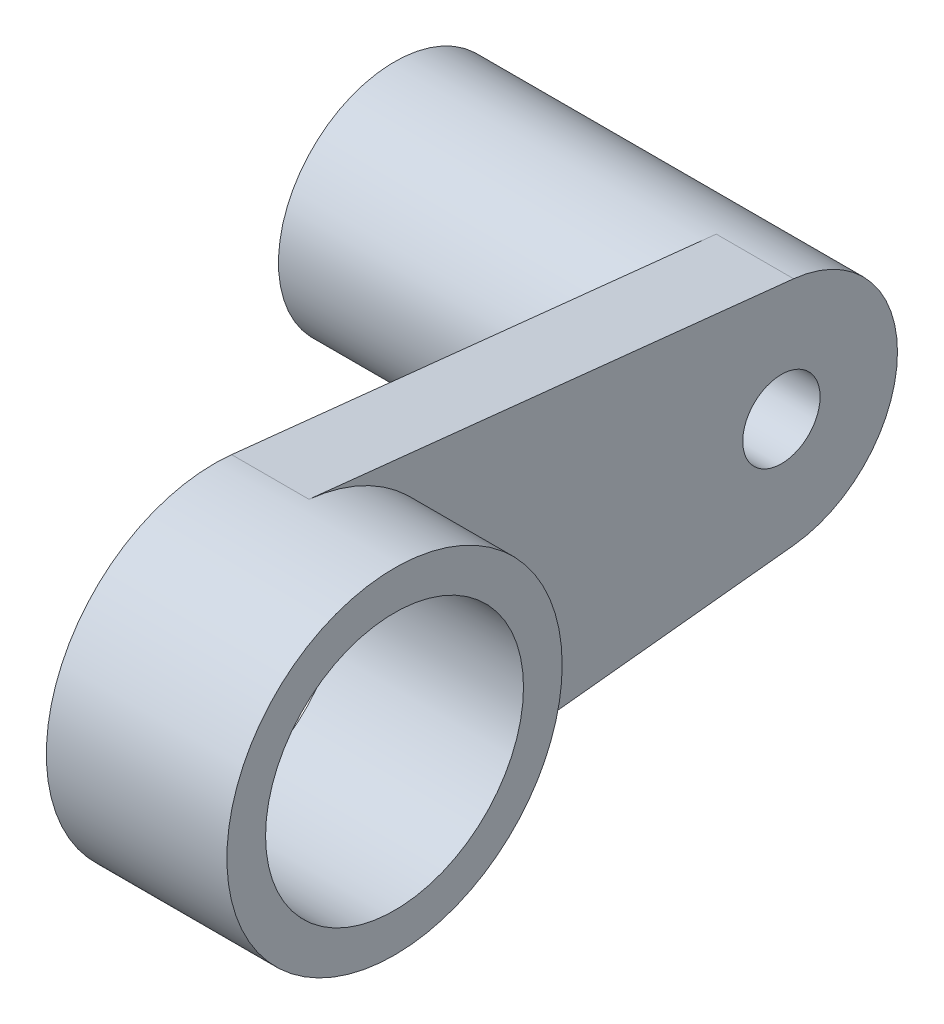
ISO-10303-21;
HEADER;
FILE_DESCRIPTION(('STEP AP214'),'2;1');
FILE_NAME('part.step','',(''),(''),'','','');
FILE_SCHEMA(('AUTOMOTIVE_DESIGN { 1 0 10303 214 1 1 1 1 }'));
ENDSEC;
DATA;
#1=APPLICATION_CONTEXT('core data for automotive mechanical design processes');
#2=APPLICATION_PROTOCOL_DEFINITION('international standard','automotive_design',2000,#1);
#3=PRODUCT_CONTEXT('',#1,'mechanical');
#4=PRODUCT('Part','Part','',(#3));
#5=PRODUCT_RELATED_PRODUCT_CATEGORY('part','',(#4));
#6=PRODUCT_DEFINITION_FORMATION('','',#4);
#7=PRODUCT_DEFINITION_CONTEXT('part definition',#1,'design');
#8=PRODUCT_DEFINITION('design','',#6,#7);
#9=PRODUCT_DEFINITION_SHAPE('','',#8);
#10=(LENGTH_UNIT() NAMED_UNIT(*) SI_UNIT(.MILLI.,.METRE.));
#11=(NAMED_UNIT(*) PLANE_ANGLE_UNIT() SI_UNIT($,.RADIAN.));
#12=(NAMED_UNIT(*) SI_UNIT($,.STERADIAN.) SOLID_ANGLE_UNIT());
#13=UNCERTAINTY_MEASURE_WITH_UNIT(LENGTH_MEASURE(1.E-05),#10,'distance_accuracy_value','');
#14=(GEOMETRIC_REPRESENTATION_CONTEXT(3) GLOBAL_UNCERTAINTY_ASSIGNED_CONTEXT((#13)) GLOBAL_UNIT_ASSIGNED_CONTEXT((#10,
#11,#12)) REPRESENTATION_CONTEXT('',''));
#15=CARTESIAN_POINT('',(0.,0.,0.));
#16=DIRECTION('',(0.,0.,1.));
#17=DIRECTION('',(1.,0.,0.));
#18=AXIS2_PLACEMENT_3D('',#15,#16,#17);
#19=CARTESIAN_POINT('',(14.,0.,0.));
#20=DIRECTION('',(-1.,0.,0.));
#21=DIRECTION('',(0.,0.,1.));
#22=AXIS2_PLACEMENT_3D('',#19,#20,#21);
#23=CYLINDRICAL_SURFACE('',#22,13.);
#24=CARTESIAN_POINT('',(14.,0.,0.));
#25=DIRECTION('',(1.,0.,0.));
#26=DIRECTION('',(0.,0.,-1.));
#27=AXIS2_PLACEMENT_3D('',#24,#25,#26);
#28=CIRCLE('',#27,13.);
#29=CARTESIAN_POINT('',(14.,0.,-13.));
#30=VERTEX_POINT('',#29);
#31=EDGE_CURVE('E11',#30,#30,#28,.T.);
#32=ORIENTED_EDGE('',*,*,#31,.F.);
#33=EDGE_LOOP('',(#32));
#34=FACE_BOUND('',#33,.T.);
#35=DIRECTION('',(-1.,0.,0.));
#36=VECTOR('',#35,1.);
#37=CARTESIAN_POINT('',(6.,-12.9277772189466,-1.36842105263158));
#38=LINE('',#37,#36);
#39=CARTESIAN_POINT('',(6.,-12.9277772189466,-1.36842105263158));
#40=VERTEX_POINT('',#39);
#41=CARTESIAN_POINT('',(0.,-12.9277772189466,-1.36842105263158));
#42=VERTEX_POINT('',#41);
#43=EDGE_CURVE('E63',#40,#42,#38,.T.);
#44=ORIENTED_EDGE('',*,*,#43,.F.);
#45=CARTESIAN_POINT('',(6.,0.,0.));
#46=DIRECTION('',(1.,0.,0.));
#47=DIRECTION('',(0.,0.,-1.));
#48=AXIS2_PLACEMENT_3D('',#45,#46,#47);
#49=CIRCLE('',#48,13.);
#50=CARTESIAN_POINT('',(6.,12.9277772189466,-1.36842105263158));
#51=VERTEX_POINT('',#50);
#52=EDGE_CURVE('E59',#40,#51,#49,.T.);
#53=ORIENTED_EDGE('',*,*,#52,.T.);
#54=DIRECTION('',(-1.,0.,0.));
#55=VECTOR('',#54,1.);
#56=CARTESIAN_POINT('',(6.,12.9277772189466,-1.36842105263158));
#57=LINE('',#56,#55);
#58=CARTESIAN_POINT('',(0.,12.9277772189466,-1.36842105263158));
#59=VERTEX_POINT('',#58);
#60=EDGE_CURVE('E111',#51,#59,#57,.T.);
#61=ORIENTED_EDGE('',*,*,#60,.T.);
#62=CARTESIAN_POINT('',(0.,0.,0.));
#63=DIRECTION('',(1.,0.,0.));
#64=DIRECTION('',(0.,0.,-1.));
#65=AXIS2_PLACEMENT_3D('',#62,#63,#64);
#66=CIRCLE('',#65,13.);
#67=EDGE_CURVE('E116',#59,#42,#66,.T.);
#68=ORIENTED_EDGE('',*,*,#67,.T.);
#69=EDGE_LOOP('',(#44,#53,#61,#68));
#70=FACE_BOUND('',#69,.T.);
#71=ADVANCED_FACE('F41',(#34,#70),#23,.T.);
#72=CARTESIAN_POINT('',(14.,0.,0.));
#73=DIRECTION('',(-1.,0.,0.));
#74=DIRECTION('',(0.,0.,1.));
#75=AXIS2_PLACEMENT_3D('',#72,#73,#74);
#76=CYLINDRICAL_SURFACE('',#75,10.);
#77=CARTESIAN_POINT('',(14.,0.,0.));
#78=DIRECTION('',(1.,0.,0.));
#79=DIRECTION('',(0.,0.,-1.));
#80=AXIS2_PLACEMENT_3D('',#77,#78,#79);
#81=CIRCLE('',#80,10.);
#82=CARTESIAN_POINT('',(14.,0.,-10.));
#83=VERTEX_POINT('',#82);
#84=EDGE_CURVE('E49',#83,#83,#81,.T.);
#85=ORIENTED_EDGE('',*,*,#84,.T.);
#86=EDGE_LOOP('',(#85));
#87=FACE_BOUND('',#86,.T.);
#88=CARTESIAN_POINT('',(0.,0.,0.));
#89=DIRECTION('',(1.,0.,0.));
#90=DIRECTION('',(0.,0.,-1.));
#91=AXIS2_PLACEMENT_3D('',#88,#89,#90);
#92=CIRCLE('',#91,10.);
#93=CARTESIAN_POINT('',(0.,0.,-10.));
#94=VERTEX_POINT('',#93);
#95=EDGE_CURVE('E118',#94,#94,#92,.T.);
#96=ORIENTED_EDGE('',*,*,#95,.F.);
#97=EDGE_LOOP('',(#96));
#98=FACE_BOUND('',#97,.T.);
#99=ADVANCED_FACE('F43',(#87,#98),#76,.F.);
#100=CARTESIAN_POINT('',(14.,0.,0.));
#101=DIRECTION('',(1.,0.,0.));
#102=DIRECTION('',(0.,0.,-1.));
#103=AXIS2_PLACEMENT_3D('',#100,#101,#102);
#104=PLANE('',#103);
#105=ORIENTED_EDGE('',*,*,#84,.F.);
#106=EDGE_LOOP('',(#105));
#107=FACE_BOUND('',#106,.T.);
#108=ORIENTED_EDGE('',*,*,#31,.T.);
#109=EDGE_LOOP('',(#108));
#110=FACE_BOUND('',#109,.T.);
#111=ADVANCED_FACE('F160',(#107,#110),#104,.T.);
#112=CARTESIAN_POINT('',(0.,0.,0.));
#113=DIRECTION('',(1.,0.,0.));
#114=DIRECTION('',(0.,0.,-1.));
#115=AXIS2_PLACEMENT_3D('',#112,#113,#114);
#116=PLANE('',#115);
#117=ORIENTED_EDGE('',*,*,#95,.T.);
#118=EDGE_LOOP('',(#117));
#119=FACE_BOUND('',#118,.T.);
#120=DIRECTION('',(0.,-0.105263157894737,-0.994444401457431));
#121=VECTOR('',#120,1.);
#122=CARTESIAN_POINT('',(0.,12.9277772189466,-1.36842105263158));
#123=LINE('',#122,#121);
#124=CARTESIAN_POINT('',(0.,8.94999961311688,-38.9473684210526));
#125=VERTEX_POINT('',#124);
#126=EDGE_CURVE('E90',#59,#125,#123,.T.);
#127=ORIENTED_EDGE('',*,*,#126,.T.);
#128=CARTESIAN_POINT('',(0.,0.,-38.));
#129=DIRECTION('',(1.,0.,0.));
#130=DIRECTION('',(0.,0.,-1.));
#131=AXIS2_PLACEMENT_3D('',#128,#129,#130);
#132=CIRCLE('',#131,9.);
#133=CARTESIAN_POINT('',(0.,-8.94999961311688,-38.9473684210526));
#134=VERTEX_POINT('',#133);
#135=EDGE_CURVE('E82',#125,#134,#132,.T.);
#136=ORIENTED_EDGE('',*,*,#135,.T.);
#137=DIRECTION('',(0.,-0.105263157894737,0.994444401457431));
#138=VECTOR('',#137,1.);
#139=CARTESIAN_POINT('',(0.,-12.9277772189466,-1.36842105263158));
#140=LINE('',#139,#138);
#141=EDGE_CURVE('E87',#134,#42,#140,.T.);
#142=ORIENTED_EDGE('',*,*,#141,.T.);
#143=ORIENTED_EDGE('',*,*,#67,.F.);
#144=EDGE_LOOP('',(#127,#136,#142,#143));
#145=FACE_BOUND('',#144,.T.);
#146=ADVANCED_FACE('F81',(#119,#145),#116,.F.);
#147=CARTESIAN_POINT('',(6.,-12.9277772189466,-1.36842105263158));
#148=DIRECTION('',(0.,-0.994444401457431,-0.105263157894737));
#149=DIRECTION('',(0.,0.105263157894737,-0.994444401457431));
#150=AXIS2_PLACEMENT_3D('',#147,#148,#149);
#151=PLANE('',#150);
#152=ORIENTED_EDGE('',*,*,#141,.F.);
#153=DIRECTION('',(-1.,0.,0.));
#154=VECTOR('',#153,1.);
#155=CARTESIAN_POINT('',(6.,-8.94999961311688,-38.9473684210526));
#156=LINE('',#155,#154);
#157=CARTESIAN_POINT('',(6.,-8.94999961311688,-38.9473684210526));
#158=VERTEX_POINT('',#157);
#159=EDGE_CURVE('E96',#158,#134,#156,.T.);
#160=ORIENTED_EDGE('',*,*,#159,.F.);
#161=DIRECTION('',(0.,-0.105263157894737,0.994444401457431));
#162=VECTOR('',#161,1.);
#163=CARTESIAN_POINT('',(6.,-12.9277772189466,-1.36842105263158));
#164=LINE('',#163,#162);
#165=EDGE_CURVE('E126',#158,#40,#164,.T.);
#166=ORIENTED_EDGE('',*,*,#165,.T.);
#167=ORIENTED_EDGE('',*,*,#43,.T.);
#168=EDGE_LOOP('',(#152,#160,#166,#167));
#169=FACE_BOUND('',#168,.T.);
#170=ADVANCED_FACE('F104',(#169),#151,.T.);
#171=CARTESIAN_POINT('',(6.,0.,-38.));
#172=DIRECTION('',(-1.,0.,0.));
#173=DIRECTION('',(0.,0.,1.));
#174=AXIS2_PLACEMENT_3D('',#171,#172,#173);
#175=CYLINDRICAL_SURFACE('',#174,9.);
#176=ORIENTED_EDGE('',*,*,#159,.T.);
#177=ORIENTED_EDGE('',*,*,#135,.F.);
#178=DIRECTION('',(-1.,0.,0.));
#179=VECTOR('',#178,1.);
#180=CARTESIAN_POINT('',(6.,8.94999961311688,-38.9473684210526));
#181=LINE('',#180,#179);
#182=CARTESIAN_POINT('',(6.,8.94999961311688,-38.9473684210526));
#183=VERTEX_POINT('',#182);
#184=EDGE_CURVE('E103',#183,#125,#181,.T.);
#185=ORIENTED_EDGE('',*,*,#184,.F.);
#186=CARTESIAN_POINT('',(6.,0.,-38.));
#187=DIRECTION('',(1.,0.,0.));
#188=DIRECTION('',(0.,0.,-1.));
#189=AXIS2_PLACEMENT_3D('',#186,#187,#188);
#190=CIRCLE('',#189,9.);
#191=EDGE_CURVE('E97',#158,#183,#190,.T.);
#192=ORIENTED_EDGE('',*,*,#191,.F.);
#193=EDGE_LOOP('',(#176,#177,#185,#192));
#194=FACE_BOUND('',#193,.T.);
#195=CARTESIAN_POINT('',(-24.,0.,-38.));
#196=DIRECTION('',(1.,0.,0.));
#197=DIRECTION('',(0.,0.,-1.));
#198=AXIS2_PLACEMENT_3D('',#195,#196,#197);
#199=CIRCLE('',#198,9.);
#200=CARTESIAN_POINT('',(-24.,0.,-47.));
#201=VERTEX_POINT('',#200);
#202=EDGE_CURVE('E91',#201,#201,#199,.T.);
#203=ORIENTED_EDGE('',*,*,#202,.T.);
#204=EDGE_LOOP('',(#203));
#205=FACE_BOUND('',#204,.T.);
#206=ADVANCED_FACE('F100',(#194,#205),#175,.T.);
#207=CARTESIAN_POINT('',(6.,12.9277772189466,-1.36842105263158));
#208=DIRECTION('',(0.,0.994444401457431,-0.105263157894737));
#209=DIRECTION('',(0.,0.105263157894737,0.994444401457431));
#210=AXIS2_PLACEMENT_3D('',#207,#208,#209);
#211=PLANE('',#210);
#212=ORIENTED_EDGE('',*,*,#126,.F.);
#213=ORIENTED_EDGE('',*,*,#60,.F.);
#214=DIRECTION('',(0.,-0.105263157894737,-0.994444401457431));
#215=VECTOR('',#214,1.);
#216=CARTESIAN_POINT('',(6.,12.9277772189466,-1.36842105263158));
#217=LINE('',#216,#215);
#218=EDGE_CURVE('E112',#51,#183,#217,.T.);
#219=ORIENTED_EDGE('',*,*,#218,.T.);
#220=ORIENTED_EDGE('',*,*,#184,.T.);
#221=EDGE_LOOP('',(#212,#213,#219,#220));
#222=FACE_BOUND('',#221,.T.);
#223=ADVANCED_FACE('F127',(#222),#211,.T.);
#224=CARTESIAN_POINT('',(6.,0.,0.));
#225=DIRECTION('',(1.,0.,0.));
#226=DIRECTION('',(0.,0.,-1.));
#227=AXIS2_PLACEMENT_3D('',#224,#225,#226);
#228=PLANE('',#227);
#229=CARTESIAN_POINT('',(6.,0.,-38.));
#230=DIRECTION('',(1.,0.,0.));
#231=DIRECTION('',(0.,0.,-1.));
#232=AXIS2_PLACEMENT_3D('',#229,#230,#231);
#233=CIRCLE('',#232,3.);
#234=CARTESIAN_POINT('',(6.,0.,-41.));
#235=VERTEX_POINT('',#234);
#236=EDGE_CURVE('E135',#235,#235,#233,.T.);
#237=ORIENTED_EDGE('',*,*,#236,.F.);
#238=EDGE_LOOP('',(#237));
#239=FACE_BOUND('',#238,.T.);
#240=ORIENTED_EDGE('',*,*,#52,.F.);
#241=ORIENTED_EDGE('',*,*,#165,.F.);
#242=ORIENTED_EDGE('',*,*,#191,.T.);
#243=ORIENTED_EDGE('',*,*,#218,.F.);
#244=EDGE_LOOP('',(#240,#241,#242,#243));
#245=FACE_BOUND('',#244,.T.);
#246=ADVANCED_FACE('F146',(#239,#245),#228,.T.);
#247=CARTESIAN_POINT('',(-24.,0.,-38.));
#248=DIRECTION('',(1.,0.,0.));
#249=DIRECTION('',(0.,0.,-1.));
#250=AXIS2_PLACEMENT_3D('',#247,#248,#249);
#251=PLANE('',#250);
#252=CARTESIAN_POINT('',(-24.,0.,-38.));
#253=DIRECTION('',(1.,0.,0.));
#254=DIRECTION('',(0.,0.,-1.));
#255=AXIS2_PLACEMENT_3D('',#252,#253,#254);
#256=CIRCLE('',#255,3.);
#257=CARTESIAN_POINT('',(-24.,0.,-41.));
#258=VERTEX_POINT('',#257);
#259=EDGE_CURVE('E44',#258,#258,#256,.T.);
#260=ORIENTED_EDGE('',*,*,#259,.T.);
#261=EDGE_LOOP('',(#260));
#262=FACE_BOUND('',#261,.T.);
#263=ORIENTED_EDGE('',*,*,#202,.F.);
#264=EDGE_LOOP('',(#263));
#265=FACE_BOUND('',#264,.T.);
#266=ADVANCED_FACE('F140',(#262,#265),#251,.F.);
#267=CARTESIAN_POINT('',(-31.,0.,-38.));
#268=DIRECTION('',(1.,0.,0.));
#269=DIRECTION('',(0.,0.,-1.));
#270=AXIS2_PLACEMENT_3D('',#267,#268,#269);
#271=CYLINDRICAL_SURFACE('',#270,3.);
#272=ORIENTED_EDGE('',*,*,#236,.T.);
#273=EDGE_LOOP('',(#272));
#274=FACE_BOUND('',#273,.T.);
#275=ORIENTED_EDGE('',*,*,#259,.F.);
#276=EDGE_LOOP('',(#275));
#277=FACE_BOUND('',#276,.T.);
#278=ADVANCED_FACE('F142',(#274,#277),#271,.F.);
#279=CLOSED_SHELL('',(#71,#99,#111,#146,#170,#206,#223,#246,#266,#278));
#280=MANIFOLD_SOLID_BREP('B2',#279);
#281=ADVANCED_BREP_SHAPE_REPRESENTATION('',(#18,#280),#14);
#282=SHAPE_DEFINITION_REPRESENTATION(#9,#281);
ENDSEC;
END-ISO-10303-21;
